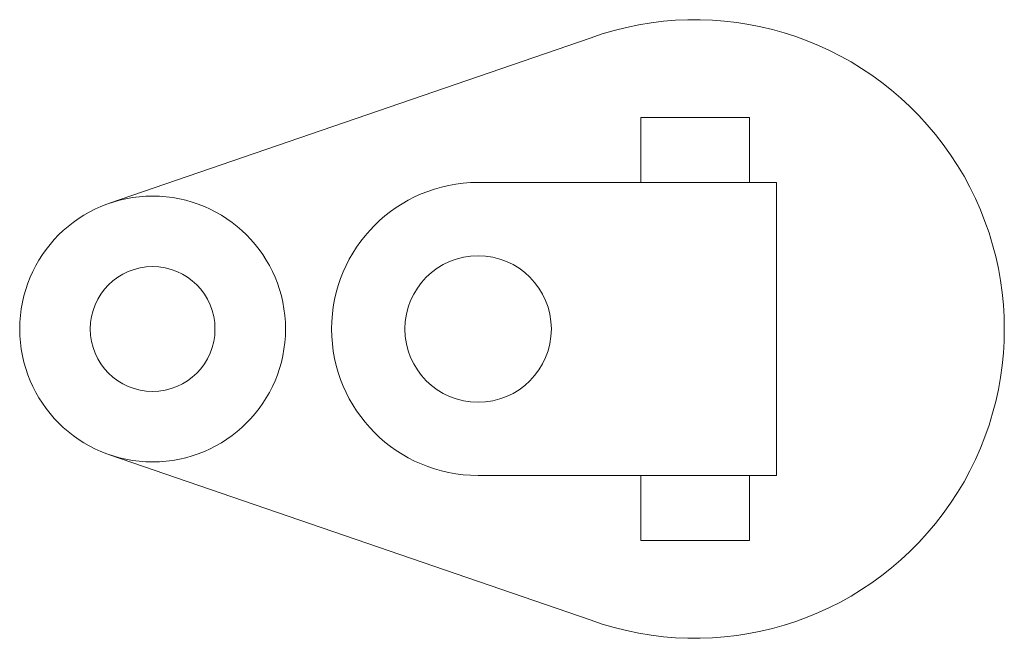
# Model space of a CAD drawing. Units: millimetres. Extents: x 2306 to 2487, y 1414 to 1528.
import ezdxf

# ---------------------------------------------------------------- set-up
doc = ezdxf.new("R2010")
doc.units = ezdxf.units.MM
doc.layers.add('M-CONS', color=8, linetype='Continuous', lineweight=18)

msp = doc.modelspace()

# ---------------------------------------------------------------- linework, layer by layer
at = {"layer": 'M-CONS'}
msp.add_line((2445.04, 1470.73), (2445.04, 1497.73), dxfattribs=at)
for points in [[(2322.08, 1493.9), (2410.68, 1524.34, -1.424173), (2410.68, 1417.11), (2322.08, 1447.56)], [(2440.04, 1497.73), (2440.04, 1500.2), (2440.04, 1497.73), (2390.04, 1497.73, 1), (2390.04, 1443.73), (2440.04, 1443.73), (2445.04, 1443.73), (2445.04, 1497.73), (2440.04, 1497.73), (2440.04, 1509.73), (2420.04, 1509.73), (2420.04, 1497.73)]]:
    msp.add_lwpolyline(points, format="xyb", dxfattribs=at)
msp.add_lwpolyline([(2440.04, 1437.16), (2440.04, 1443.73), (2440.04, 1431.73), (2420.04, 1431.73), (2420.04, 1443.73)], dxfattribs=at)
at = {"layer": 'M-CONS', "extrusion": (0, 1, 0)}
for radius in [10, 6]:
    msp.add_circle((-2430.04, 63, 1509.73), radius, dxfattribs=at)
at = {"layer": 'M-CONS'}
for centre, radius in [((2330.04, 1470.73), 24.5), ((2390.04, 1470.73), 13.5), ((2330.04, 1470.73), 11.5)]:
    msp.add_circle(centre, radius, dxfattribs=at)
at = {"layer": 'M-CONS', "extrusion": (0, -1, 0)}
for radius in [10, 6]:
    msp.add_circle((2430.04, 63, -1431.73), radius, dxfattribs=at)

doc.saveas('drawing.dxf')
